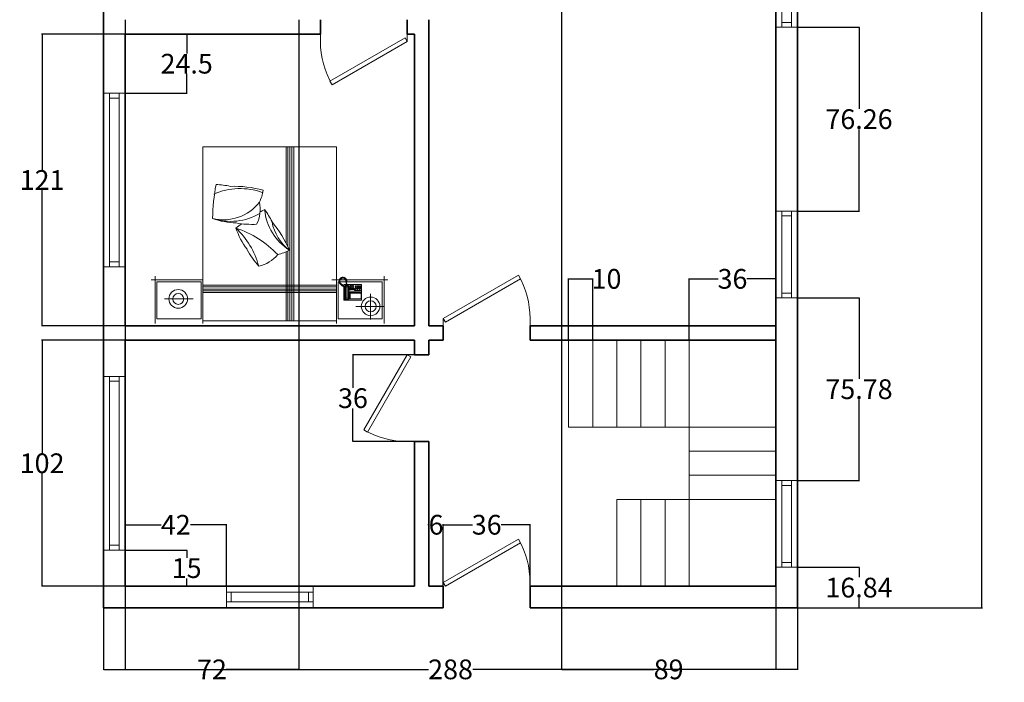
# Model space of a CAD drawing. Units: inches. Extents: x -254 to 1961, y 86 to 3025.
# Tile 2 of 6: x 117 to 525, y 133 to 408. Entities that reach past the tile are written whole.
import ezdxf

# ---------------------------------------------------------------- set-up
doc = ezdxf.new("R2010")
doc.units = ezdxf.units.IN
doc.header["$MEASUREMENT"] = 0
for name, color, linetype, lineweight in [('A-ANNO-DIMS', 2, 'Continuous', 18), ('DOORS', 40, 'Continuous', 18), ('FURNITURE', 151, 'Continuous', 13), ('STAIRCASE', 212, 'Continuous', 18), ('WALLS', 255, 'Continuous', 35), ('WINDOWS', 50, 'Continuous', 18)]:
    doc.layers.add(name, color=color, linetype=linetype, lineweight=lineweight)
doc.styles.get("Standard").update_dxf_attribs({"font": 'arial.ttf'})
doc.dimstyles.get("Standard").update_dxf_attribs({"dimtxt": 8.18, "dimasz": 0.18, "dimexe": 0.18, "dimexo": 0.0625, "dimgap": 0.09, "dimtad": 0, "dimtih": 1, "dimtoh": 1, "dimdec": 1, "dimzin": 0, "dimdsep": 46, "dimlunit": 3, "dimtxsty": 'Standard', "dimcen": 0.09, "dimadec": 0, "dimazin": 0, "dimtfac": 1, "dimtdec": 1, "dimtofl": 0, "dimtmove": 0, "dimatfit": 3, "dimfxl": 1, "dimtolj": 1, "dimtzin": 0, "dimarcsym": 0})

# ---------------------------------------------------------------- blocks, each defined once
blk = doc.blocks.new('*U5')
for p, q in [((0, 0), (0, -6)), ((36, 0), (36, -6))]:
    blk.add_line(p, q)
blk.add_lwpolyline([(0, 0), (31.18, 18), (32.05, 16.48), (0.87, -1.52)], close=True)
blk.add_arc((0, 0), 36, 0, 30)
blk = doc.blocks.new('*U3')
for p, q in [((-36, 0), (-36, 6)), ((0, 0), (0, 6))]:
    blk.add_line(p, q)
blk.add_lwpolyline([(0, 0), (-31.18, -18), (-32.05, -16.48), (-0.88, 1.52)], close=True)
blk.add_arc((0, 0), 36, 180, 210)
blk = doc.blocks.new('*U7')
for p, q in [((0, 0), (0, -6)), ((-36, 0), (-36, -6))]:
    blk.add_line(p, q)
blk.add_lwpolyline([(0, 0), (-31.18, 18), (-32.05, 16.48), (-0.88, -1.52)], close=True)
blk.add_arc((0, 0), 36, 150, 180)
blk = doc.blocks.new('BED-DOUBLE-NIGHTSTANDS')
for p, q in [((1.58, 73.32), (1.58, 53.78)), ((20.68, 71.37), (2.35, 71.37)), ((2.35, 71.37), (2.35, 56.1)), ((20.68, 56.1), (20.68, 71.37)), ((21.4, 73.32), (21.4, 53.78)), ((76.84, 72.19), (21.4, 72.19)), ((21.4, 72.19), (21.4, 0)), ((55.98, 43.63), (55.98, 72.19)), ((56.73, 43.3), (56.73, 72.19)), ((57.47, 0), (57.47, 72.19)), ((58.37, 0), (58.37, 72.19)), ((59.13, 0), (59.13, 72.19)), ((76.84, 73.32), (76.84, 53.78)), ((76.84, 0), (76.84, 72.19)), ((77.56, 56.1), (77.56, 71.37)), ((77.56, 71.37), (95.89, 71.37)), ((91.03, 61.02), (91.03, 71.64)), ((95.89, 71.37), (95.89, 56.1)), ((96.61, 73.32), (96.61, 53.78)), ((96.71, 66.24), (84.84, 66.24)), ((5.54, 63.15), (17.4, 63.15)), ((79.99, 63.51), (80.08, 63.61)), ((79.99, 57.27), (79.99, 63.51)), ((80.08, 63.61), (87.23, 63.61)), ((80.58, 63.47), (80.35, 63.24)), ((80.35, 63.24), (80.35, 57.81)), ((80.49, 63.33), (80.44, 63.15)), ((80.85, 62.75), (80.44, 63.15)), ((80.44, 63.15), (80.44, 61.93)), ((80.44, 61.93), (80.54, 61.7)), ((80.67, 63.42), (80.49, 63.33)), ((80.54, 61.7), (80.67, 61.48)), ((81.94, 63.47), (80.58, 63.47)), ((81.76, 63.42), (80.67, 63.42)), ((80.9, 62.84), (80.67, 63.42)), ((80.67, 61.48), (80.72, 61.16)), ((80.9, 62.84), (80.85, 62.75)), ((80.85, 62.75), (80.85, 60.71)), ((81.53, 62.84), (80.9, 62.84)), ((81.76, 63.42), (81.53, 62.84)), ((81.58, 62.75), (81.53, 62.84)), ((81.98, 63.15), (81.58, 62.75)), ((81.58, 62.75), (81.58, 60.71)), ((81.71, 61.16), (81.76, 61.48)), ((81.94, 63.33), (81.76, 63.42)), ((81.76, 61.48), (81.89, 61.7)), ((81.89, 61.7), (81.98, 61.93)), ((82.12, 63.24), (81.94, 63.47)), ((81.98, 63.15), (81.94, 63.33)), ((81.98, 61.93), (81.98, 63.15)), ((82.12, 57.77), (82.12, 63.24)), ((82.53, 60.71), (82.53, 63.11)), ((82.53, 63.11), (87.05, 63.11)), ((87.05, 63.11), (87.05, 60.71)), ((87.23, 63.61), (87.32, 63.51)), ((87.32, 63.51), (87.32, 57.27)), ((21.4, 60.55), (76.84, 60.55)), ((21.4, 59.81), (76.84, 59.81)), ((21.4, 59.06), (76.84, 59.06)), ((21.4, 58.17), (76.84, 58.17)), ((21.4, 57.41), (76.84, 57.41)), ((79.19, 57.22), (78.6, 56.71)), ((78.72, 57.24), (78.93, 57.44)), ((78.77, 56.95), (78.72, 57.24)), ((78.93, 57.44), (79.18, 57.31)), ((79.08, 57.58), (79.2, 57.7)), ((79.18, 57.31), (79.08, 57.58)), ((79.56, 57.55), (79.19, 57.22)), ((79.2, 57.7), (79.31, 57.62)), ((79.25, 57.75), (79.33, 57.83)), ((79.31, 57.62), (79.25, 57.75)), ((79.33, 57.83), (79.5, 57.77)), ((79.56, 57.64), (79.47, 57.65)), ((79.47, 57.65), (79.56, 57.55)), ((79.5, 57.77), (79.59, 57.85)), ((79.61, 57.7), (79.56, 57.64)), ((79.59, 57.85), (79.72, 57.98)), ((79.79, 57.85), (79.61, 57.7)), ((79.72, 57.98), (79.99, 58.08)), ((79.99, 57.9), (79.79, 57.85)), ((80.08, 57.18), (79.99, 57.27)), ((80.35, 57.81), (80.58, 57.54)), ((80.54, 59.31), (80.44, 59.08)), ((80.44, 59.08), (80.44, 57.86)), ((80.44, 57.86), (80.85, 58.26)), ((80.49, 57.68), (80.44, 57.86)), ((80.67, 57.59), (80.49, 57.68)), ((80.67, 59.53), (80.54, 59.31)), ((80.58, 57.54), (81.11, 57.54)), ((80.72, 59.85), (80.67, 59.53)), ((80.67, 57.59), (80.9, 58.17)), ((81.11, 57.59), (80.67, 57.59)), ((80.72, 61.16), (80.72, 60.71)), ((80.72, 60.71), (80.72, 59.85)), ((80.85, 60.71), (80.85, 58.26)), ((80.85, 58.26), (80.9, 58.17)), ((80.9, 58.17), (81.53, 58.17)), ((81.03, 57.07), (81.1, 57.36)), ((81.1, 57.36), (81.12, 57.72)), ((81.12, 57.72), (81.26, 57.72)), ((81.25, 57.33), (81.14, 56.87)), ((81.26, 57.72), (81.25, 57.33)), ((81.76, 57.59), (81.26, 57.59)), ((81.26, 57.54), (81.89, 57.54)), ((81.58, 58.26), (81.53, 58.17)), ((81.53, 58.17), (81.76, 57.59)), ((81.58, 60.71), (81.58, 58.26)), ((81.98, 57.86), (81.58, 58.26)), ((81.71, 60.71), (81.71, 61.16)), ((81.71, 59.85), (81.71, 60.71)), ((82.12, 60.34), (81.71, 60.34)), ((81.76, 59.53), (81.71, 59.85)), ((81.89, 59.31), (81.76, 59.53)), ((81.76, 57.59), (81.94, 57.68)), ((81.98, 59.08), (81.89, 59.31)), ((81.89, 57.54), (82.12, 57.77)), ((81.94, 57.68), (81.98, 57.86)), ((81.98, 57.86), (81.98, 59.08)), ((87.05, 60.71), (82.53, 60.71)), ((82.53, 60.17), (82.53, 60.62)), ((82.53, 60.62), (86.87, 60.62)), ((86.87, 60.34), (82.53, 60.34)), ((86.87, 60.17), (82.53, 60.17)), ((82.89, 59.44), (82.53, 59.44)), ((82.53, 59.44), (82.53, 59.17)), ((82.53, 59.17), (82.89, 59.17)), ((82.89, 58.94), (82.53, 58.94)), ((82.53, 58.94), (82.53, 58.67)), ((82.53, 58.67), (82.89, 58.67)), ((82.53, 58.45), (82.53, 58.17)), ((82.89, 58.45), (82.53, 58.45)), ((82.53, 58.17), (82.89, 58.17)), ((82.53, 57.9), (82.53, 57.63)), ((82.89, 57.9), (82.53, 57.9)), ((82.53, 57.63), (82.89, 57.63)), ((82.89, 59.17), (82.89, 59.44)), ((82.89, 58.67), (82.89, 58.94)), ((82.89, 58.17), (82.89, 58.45)), ((82.89, 57.63), (82.89, 57.9)), ((83.07, 59.44), (83.07, 59.17)), ((83.43, 59.44), (83.07, 59.44)), ((83.07, 59.17), (83.43, 59.17)), ((83.43, 58.94), (83.07, 58.94)), ((83.07, 58.94), (83.07, 58.67)), ((83.07, 58.67), (83.43, 58.67)), ((83.07, 58.4), (83.07, 58.13)), ((83.43, 58.4), (83.07, 58.4)), ((83.07, 58.13), (83.43, 58.13)), ((83.43, 57.9), (83.07, 57.9)), ((83.07, 57.9), (83.07, 57.63)), ((83.07, 57.63), (83.43, 57.63)), ((83.43, 59.17), (83.43, 59.44)), ((83.43, 58.67), (83.43, 58.94)), ((83.43, 58.13), (83.43, 58.4)), ((83.43, 57.63), (83.43, 57.9)), ((83.97, 59.44), (83.61, 59.44)), ((83.61, 59.44), (83.61, 59.17)), ((83.61, 59.17), (83.97, 59.17)), ((83.97, 58.94), (83.61, 58.94)), ((83.61, 58.94), (83.61, 58.67)), ((83.61, 58.67), (83.97, 58.67)), ((83.97, 58.4), (83.61, 58.4)), ((83.61, 58.4), (83.61, 58.13)), ((83.61, 58.13), (83.97, 58.13)), ((83.97, 57.9), (83.61, 57.9)), ((83.61, 57.9), (83.61, 57.63)), ((83.61, 57.63), (83.97, 57.63)), ((83.97, 59.17), (83.97, 59.44)), ((83.97, 58.67), (83.97, 58.94)), ((83.97, 58.13), (83.97, 58.4)), ((83.97, 57.63), (83.97, 57.9)), ((84.38, 58.85), (84.38, 59.67)), ((84.38, 59.67), (87.05, 59.67)), ((87.05, 58.85), (84.38, 58.85)), ((84.73, 60.17), (84.56, 60.34)), ((84.65, 58.45), (84.65, 58.63)), ((84.65, 58.63), (85.11, 58.63)), ((85.11, 58.45), (84.65, 58.45)), ((85.11, 57.95), (84.65, 57.95)), ((84.65, 57.95), (84.65, 57.68)), ((84.65, 57.68), (85.11, 57.68)), ((84.7, 60.62), (84.7, 60.17)), ((84.83, 59.44), (84.83, 59.58)), ((84.83, 59.58), (84.97, 59.58)), ((84.97, 59.44), (84.83, 59.44)), ((84.83, 58.94), (84.83, 59.08)), ((84.83, 59.08), (84.97, 59.08)), ((84.97, 58.94), (84.83, 58.94)), ((84.97, 59.58), (84.97, 59.44)), ((84.97, 59.08), (84.97, 58.94)), ((85.06, 60.62), (85.06, 60.17)), ((85.11, 58.63), (85.11, 58.45)), ((85.11, 57.68), (85.11, 57.95)), ((86.04, 58.85), (85.23, 59.67)), ((85.29, 58.63), (85.74, 58.63)), ((85.29, 58.45), (85.29, 58.63)), ((85.74, 58.45), (85.29, 58.45)), ((85.29, 57.95), (85.29, 57.68)), ((85.74, 57.95), (85.29, 57.95)), ((85.29, 57.68), (85.74, 57.68)), ((85.42, 60.62), (85.42, 60.17)), ((85.65, 59.44), (85.65, 59.58)), ((85.65, 59.58), (85.79, 59.58)), ((85.79, 59.44), (85.65, 59.44)), ((85.65, 58.94), (85.65, 59.08)), ((85.65, 59.08), (85.79, 59.08)), ((85.79, 58.94), (85.65, 58.94)), ((85.74, 58.63), (85.74, 58.45)), ((85.74, 57.68), (85.74, 57.95)), ((85.79, 60.62), (85.79, 60.17)), ((85.79, 59.58), (85.79, 59.44)), ((85.79, 59.08), (85.79, 58.94)), ((85.92, 58.63), (86.37, 58.63)), ((85.92, 58.45), (85.92, 58.63)), ((86.37, 58.45), (85.92, 58.45)), ((85.92, 57.95), (85.92, 57.68)), ((86.37, 57.95), (85.92, 57.95)), ((85.92, 57.68), (86.37, 57.68)), ((86.15, 60.62), (86.15, 60.17)), ((86.37, 58.52), (86.27, 58.63)), ((86.37, 58.63), (86.37, 58.45)), ((86.37, 57.68), (86.37, 57.95)), ((86.46, 59.44), (86.46, 59.58)), ((86.46, 59.58), (86.6, 59.58)), ((86.6, 59.44), (86.46, 59.44)), ((86.46, 58.94), (86.46, 59.08)), ((86.46, 59.08), (86.6, 59.08)), ((86.6, 58.94), (86.46, 58.94)), ((86.51, 60.62), (86.51, 60.17)), ((86.55, 58.63), (87.01, 58.63)), ((86.55, 58.45), (86.55, 58.63)), ((87.01, 58.45), (86.55, 58.45)), ((86.55, 57.95), (86.55, 57.68)), ((87.01, 57.95), (86.55, 57.95)), ((86.55, 57.68), (87.01, 57.68)), ((86.6, 59.58), (86.6, 59.44)), ((86.6, 59.08), (86.6, 58.94)), ((86.87, 60.62), (86.87, 60.17)), ((87.01, 57.89), (86.95, 57.95)), ((87.01, 58.63), (87.01, 58.45)), ((87.01, 57.68), (87.01, 57.95)), ((87.05, 59.67), (87.05, 58.85)), ((87.32, 57.27), (87.23, 57.18)), ((0, 55.17), (21.4, 55.17)), ((2.35, 56.1), (20.68, 56.1)), ((98.24, 55.17), (74.88, 55.17)), ((95.89, 56.1), (77.56, 56.1)), ((77.91, 55.74), (77.96, 55.97)), ((78.19, 55.65), (77.91, 55.74)), ((77.96, 55.97), (78.2, 55.97)), ((77.96, 55.52), (78.19, 55.65)), ((77.99, 55.33), (77.96, 55.52)), ((78.28, 55.34), (77.99, 55.33)), ((78.01, 56.15), (78.07, 56.36)), ((78.2, 55.97), (78.01, 56.15)), ((78.06, 55.09), (78.28, 55.34)), ((78.13, 54.91), (78.06, 55.09)), ((78.07, 56.36), (78.37, 56.35)), ((78.1, 56.45), (78.18, 56.73)), ((78.37, 56.35), (78.1, 56.45)), ((78.4, 54.99), (78.13, 54.91)), ((78.18, 56.73), (78.46, 56.7)), ((78.38, 55.31), (78.24, 55.31)), ((78.27, 54.75), (78.4, 54.99)), ((78.39, 54.64), (78.27, 54.75)), ((78.59, 56.7), (78.29, 55.84)), ((78.29, 55.84), (78.41, 55.15)), ((78.39, 56.9), (78.56, 57.08)), ((78.46, 56.7), (78.39, 56.9)), ((78.64, 54.75), (78.39, 54.64)), ((78.41, 55.15), (78.82, 54.76)), ((78.53, 54.5), (78.64, 54.75)), ((78.68, 54.37), (78.53, 54.5)), ((78.56, 57.08), (78.77, 56.95)), ((78.87, 54.61), (78.68, 54.37)), ((78.82, 54.76), (79.35, 54.53)), ((78.84, 54.33), (78.87, 54.61)), ((78.99, 54.26), (78.84, 54.33)), ((79.2, 54.44), (78.99, 54.26)), ((79.21, 54.2), (79.2, 54.44)), ((79.38, 54.15), (79.21, 54.2)), ((79.35, 54.53), (79.9, 54.57)), ((79.49, 54.44), (79.38, 54.15)), ((79.55, 54.18), (79.49, 54.44)), ((79.71, 54.2), (79.55, 54.18)), ((79.82, 54.44), (79.71, 54.2)), ((79.93, 54.2), (79.82, 54.44)), ((79.9, 54.57), (80.38, 54.83)), ((80.13, 54.25), (79.93, 54.2)), ((81.06, 57.18), (80.08, 57.18)), ((80.32, 54.37), (80.1, 54.55)), ((80.1, 54.55), (80.13, 54.25)), ((80.49, 54.48), (80.32, 54.37)), ((80.38, 54.83), (80.73, 55.27)), ((80.67, 54.57), (80.46, 54.73)), ((80.46, 54.73), (80.49, 54.48)), ((80.8, 54.74), (80.67, 54.57)), ((80.95, 54.94), (80.68, 54.99)), ((80.68, 54.99), (80.8, 54.74)), ((80.73, 55.27), (80.78, 55.85)), ((80.74, 56.06), (80.9, 56.18)), ((80.78, 55.85), (80.74, 56.06)), ((81.11, 55.38), (80.81, 55.35)), ((80.81, 55.35), (81.07, 55.15)), ((81.13, 55.83), (80.87, 55.78)), ((80.87, 55.78), (81.12, 55.63)), ((80.9, 56.41), (80.92, 56.63)), ((80.9, 56.18), (80.9, 56.41)), ((80.92, 56.63), (81.03, 57.07)), ((81.07, 55.15), (80.95, 54.94)), ((81.04, 56.2), (81.01, 56.15)), ((81.01, 56.15), (81.12, 56.05)), ((81.14, 56.87), (81.03, 56.44)), ((81.03, 56.44), (81.04, 56.2)), ((81.12, 55.63), (81.11, 55.38)), ((81.12, 56.05), (81.13, 55.83)), ((87.23, 57.18), (81.22, 57.18)), ((56.73, 0), (56.73, 41.48)), ((55.98, 0), (55.98, 39.96)), ((21.4, 0), (76.84, 0))]:
    blk.add_line(p, q)
for centre, radius in [((91.03, 66.24), 3.87), ((11.21, 63.15), 3.87), ((11.21, 63.15), 2.29), ((91.03, 66.24), 2.29)]:
    blk.add_circle(centre, radius)
for centre, radius, start, end in [((11.42, 58.69), 34.44, 313.5807, 344.664), ((74.12, 23.89), 39.12, 138.9434, 151.5029), ((41.57, 35.76), 14.16, 39.5375, 77.5218), ((21.54, 74.27), 42.76, 288.5712, 316.3694), ((64.75, 23.92), 31.18, 143.3149, 161.6473), ((69.36, 24.04), 22.39, 122.3105, 174.6609), ((14.94, 61.05), 46.14, 319.6791, 336.9358), ((69.1, 27.6), 19.32, 127.3136, 169.3014), ((47.53, 23.64), 21.7, 62.9638, 76.7966), ((87.82, 103.02), 87.02, 232.7582, 234.7034), ((36.16, 0.49), 31.18, 91.7513, 110.0837), ((32.98, 6.89), 24.09, 59.8649, 108.19), ((29.97, 11.42), 18.9, 37.9983, 103.8151), ((112.46, 31.59), 87.02, 181.1946, 190.5116), ((41.96, -6.88), 39.12, 87.3798, 99.9393), ((31.02, 26.01), 14.16, 347.9738, 25.9582), ((23.83, 43.59), 29.07, 323.0649, 334.741), ((87.82, 103.02), 87.02, 240.6207, 242.0752), ((25.24, 13.81), 21.7, 11.4002, 25.233), ((36.91, 44.65), 27.26, 246.3586, 289.7064), ((26.13, 44.77), 29.07, 271.5012, 283.1774), ((34.28, 62.58), 46.14, 268.1155, 285.3722)]:
    blk.add_arc(centre, radius, start, end)
blk = doc.blocks.new('WIN-36IN')
for p, q in [((2.5, 35), (2.5, 2)), ((6.5, 35), (6.5, 2))]:
    blk.add_line(p, q)
for points in [[(0, 36), (9, 36), (9, 0), (0, 0)], [(2.5, 36), (6.5, 36), (6.5, 34), (2.5, 34)], [(2.5, 0), (6.5, 0), (6.5, 2), (2.5, 2)]]:
    blk.add_lwpolyline(points, close=True)
blk = doc.blocks.new('WIN-72IN')
for p, q in [((2.5, 70), (2.5, 2)), ((6.5, 70), (6.5, 2))]:
    blk.add_line(p, q)
for points in [[(0, 72), (9, 72), (9, 0), (0, 0)], [(2.5, 72), (6.5, 72), (6.5, 70), (2.5, 70)], [(2.5, 0), (6.5, 0), (6.5, 2), (2.5, 2)]]:
    blk.add_lwpolyline(points, close=True)
blk = doc.blocks.new('*D22')
at = {"layer": 'A-ANNO-DIMS', "color": 0, "lineweight": -2, "transparency": 16777216}
for p, q in [((151.38, 163.93), (151.38, 138.31)), ((439.38, 163.93), (439.38, 138.31)), ((151.56, 138.49), (286.18, 138.49)), ((439.2, 138.49), (304.59, 138.49))]:
    blk.add_line(p, q, dxfattribs=at)
at = {"layer": 'A-ANNO-DIMS', "color": 0, "transparency": 16777216}
for points in [[(151.56, 138.52), (151.56, 138.46), (151.38, 138.49)], [(439.2, 138.52), (439.2, 138.46), (439.38, 138.49)]]:
    blk.add_solid(points, dxfattribs=at)
at = {"layer": 'Defpoints', "color": 0, "transparency": 16777216}
for p in [(151.38, 163.99), (439.38, 163.99), (439.38, 138.49)]:
    blk.add_point(p, dxfattribs=at)
at = {"layer": 'A-ANNO-DIMS', "color": 0, "transparency": 16777216, "insert": (295.38, 138.49), "char_height": 8.18, "attachment_point": 5}
blk.add_mtext('\\A1;288', dxfattribs=at)
blk = doc.blocks.new('*D23')
at = {"layer": 'A-ANNO-DIMS', "color": 0, "lineweight": -2, "transparency": 16777216}
for p, q in [((439.44, 667.99), (516.06, 667.99)), ((515.88, 667.81), (515.88, 420.26)), ((515.88, 164.17), (515.88, 411.73)), ((439.44, 163.99), (516.06, 163.99))]:
    blk.add_line(p, q, dxfattribs=at)
at = {"layer": 'A-ANNO-DIMS', "color": 0, "transparency": 16777216}
for points in [[(515.85, 667.81), (515.91, 667.81), (515.88, 667.99)], [(515.85, 164.17), (515.91, 164.17), (515.88, 163.99)]]:
    blk.add_solid(points, dxfattribs=at)
at = {"layer": 'Defpoints', "color": 0, "transparency": 16777216}
for p in [(439.38, 667.99), (515.88, 667.99), (439.38, 163.99)]:
    blk.add_point(p, dxfattribs=at)
at = {"layer": 'A-ANNO-DIMS', "color": 0, "transparency": 16777216, "insert": (515.88, 415.99), "char_height": 8.18, "attachment_point": 5}
blk.add_mtext('\\A1;504', dxfattribs=at)
blk = doc.blocks.new('*D30')
at = {"layer": 'A-ANNO-DIMS', "color": 0, "lineweight": -2, "transparency": 16777216}
for p, q in [((160.32, 401.99), (125.7, 401.99)), ((125.88, 401.81), (125.88, 345.69)), ((125.88, 281.17), (125.88, 337.3)), ((160.32, 280.99), (125.7, 280.99))]:
    blk.add_line(p, q, dxfattribs=at)
at = {"layer": 'A-ANNO-DIMS', "color": 0, "transparency": 16777216}
for points in [[(125.85, 401.81), (125.91, 401.81), (125.88, 401.99)], [(125.85, 281.17), (125.91, 281.17), (125.88, 280.99)]]:
    blk.add_solid(points, dxfattribs=at)
at = {"layer": 'Defpoints', "color": 0, "transparency": 16777216}
for p in [(125.88, 401.99), (160.38, 401.99), (160.38, 280.99)]:
    blk.add_point(p, dxfattribs=at)
at = {"layer": 'A-ANNO-DIMS', "color": 0, "transparency": 16777216, "insert": (125.88, 341.49), "char_height": 8.18, "attachment_point": 5}
blk.add_mtext('\\A1;121', dxfattribs=at)
blk = doc.blocks.new('*D31')
at = {"layer": 'A-ANNO-DIMS', "color": 0, "lineweight": -2, "transparency": 16777216}
for p, q in [((160.32, 274.99), (125.7, 274.99)), ((125.88, 274.81), (125.88, 228.26)), ((125.88, 173.17), (125.88, 219.73)), ((160.32, 172.99), (125.7, 172.99))]:
    blk.add_line(p, q, dxfattribs=at)
at = {"layer": 'A-ANNO-DIMS', "color": 0, "transparency": 16777216}
for points in [[(125.85, 274.81), (125.91, 274.81), (125.88, 274.99)], [(125.85, 173.17), (125.91, 173.17), (125.88, 172.99)]]:
    blk.add_solid(points, dxfattribs=at)
at = {"layer": 'Defpoints', "color": 0, "transparency": 16777216}
for p in [(125.88, 274.99), (160.38, 274.99), (160.38, 172.99)]:
    blk.add_point(p, dxfattribs=at)
at = {"layer": 'A-ANNO-DIMS', "color": 0, "transparency": 16777216, "insert": (125.88, 223.99), "char_height": 8.18, "attachment_point": 5}
blk.add_mtext('\\A1;102', dxfattribs=at)
blk = doc.blocks.new('*D32')
at = {"layer": 'A-ANNO-DIMS', "color": 0, "lineweight": -2, "transparency": 16777216}
for p, q in [((160.38, 173.06), (160.38, 198.67)), ((160.56, 198.49), (175.31, 198.49)), ((202.2, 198.49), (187.45, 198.49)), ((202.38, 173.06), (202.38, 198.67))]:
    blk.add_line(p, q, dxfattribs=at)
at = {"layer": 'A-ANNO-DIMS', "color": 0, "transparency": 16777216}
for points in [[(160.56, 198.52), (160.56, 198.46), (160.38, 198.49)], [(202.2, 198.52), (202.2, 198.46), (202.38, 198.49)]]:
    blk.add_solid(points, dxfattribs=at)
at = {"layer": 'Defpoints', "color": 0, "transparency": 16777216}
for p in [(202.38, 198.49), (160.38, 172.99), (202.38, 172.99)]:
    blk.add_point(p, dxfattribs=at)
at = {"layer": 'A-ANNO-DIMS', "color": 0, "transparency": 16777216, "insert": (181.38, 198.49), "char_height": 8.18, "attachment_point": 5}
blk.add_mtext('\\A1;42', dxfattribs=at)
blk = doc.blocks.new('*D33')
at = {"layer": 'A-ANNO-DIMS', "color": 0, "lineweight": -2, "transparency": 16777216}
for p, q in [((292.38, 173.06), (292.38, 198.67)), ((292.56, 198.49), (304.44, 198.49)), ((328.2, 198.49), (316.33, 198.49)), ((328.38, 173.06), (328.38, 198.67))]:
    blk.add_line(p, q, dxfattribs=at)
at = {"layer": 'A-ANNO-DIMS', "color": 0, "transparency": 16777216}
for points in [[(292.56, 198.52), (292.56, 198.46), (292.38, 198.49)], [(328.2, 198.52), (328.2, 198.46), (328.38, 198.49)]]:
    blk.add_solid(points, dxfattribs=at)
at = {"layer": 'Defpoints', "color": 0, "transparency": 16777216}
for p in [(328.38, 198.49), (292.38, 172.99), (328.38, 172.99)]:
    blk.add_point(p, dxfattribs=at)
at = {"layer": 'A-ANNO-DIMS', "color": 0, "transparency": 16777216, "insert": (310.38, 198.49), "char_height": 8.18, "attachment_point": 5}
blk.add_mtext('\\A1;36', dxfattribs=at)
blk = doc.blocks.new('*D34')
at = {"layer": 'A-ANNO-DIMS', "color": 0, "lineweight": -2, "transparency": 16777216}
for p, q in [((286.201832, 198.494989), (286.021832, 198.494989)), ((286.381832, 173.057489), (286.381832, 198.674989)), ((292.381832, 173.057489), (292.381832, 198.674989)), ((292.561832, 198.494989), (292.741832, 198.494989))]:
    blk.add_line(p, q, dxfattribs=at)
at = {"layer": 'A-ANNO-DIMS', "color": 0, "transparency": 16777216}
for points in [[(286.201832, 198.524989), (286.201832, 198.464989), (286.381832, 198.494989)], [(292.561832, 198.524989), (292.561832, 198.464989), (292.381832, 198.494989)]]:
    blk.add_solid(points, dxfattribs=at)
at = {"layer": 'Defpoints', "color": 0, "transparency": 16777216}
for p in [(292.381832, 198.494989), (286.381832, 172.994989), (292.381832, 172.994989)]:
    blk.add_point(p, dxfattribs=at)
at = {"layer": 'A-ANNO-DIMS', "color": 0, "transparency": 16777216, "insert": (289.381832, 198.494989), "char_height": 8.18, "attachment_point": 5}
blk.add_mtext('\\A1;6', dxfattribs=at)
blk = doc.blocks.new('*D35')
at = {"layer": 'A-ANNO-DIMS', "color": 0, "lineweight": -2, "transparency": 16777216}
for p, q in [((394.38, 275.06), (394.38, 300.67)), ((394.56, 300.49), (406.44, 300.49)), ((430.2, 300.49), (418.33, 300.49)), ((430.38, 275.06), (430.38, 300.67))]:
    blk.add_line(p, q, dxfattribs=at)
at = {"layer": 'A-ANNO-DIMS', "color": 0, "transparency": 16777216}
for points in [[(394.56, 300.52), (394.56, 300.46), (394.38, 300.49)], [(430.2, 300.52), (430.2, 300.46), (430.38, 300.49)]]:
    blk.add_solid(points, dxfattribs=at)
at = {"layer": 'Defpoints', "color": 0, "transparency": 16777216}
for p in [(430.38, 300.49), (394.38, 274.99), (430.38, 274.99)]:
    blk.add_point(p, dxfattribs=at)
at = {"layer": 'A-ANNO-DIMS', "color": 0, "transparency": 16777216, "insert": (412.38, 300.49), "char_height": 8.18, "attachment_point": 5}
blk.add_mtext('\\A1;36', dxfattribs=at)
blk = doc.blocks.new('*D36')
at = {"layer": 'A-ANNO-DIMS', "color": 0, "lineweight": -2, "transparency": 16777216}
for p, q in [((160.44, 187.99), (186.06, 187.99)), ((185.88, 187.81), (185.88, 184.76)), ((185.88, 173.17), (185.88, 176.23)), ((160.44, 172.99), (186.06, 172.99))]:
    blk.add_line(p, q, dxfattribs=at)
at = {"layer": 'A-ANNO-DIMS', "color": 0, "transparency": 16777216}
for points in [[(185.85, 187.81), (185.91, 187.81), (185.88, 187.99)], [(185.85, 173.17), (185.91, 173.17), (185.88, 172.99)]]:
    blk.add_solid(points, dxfattribs=at)
at = {"layer": 'Defpoints', "color": 0, "transparency": 16777216}
for p in [(160.38, 187.99), (160.38, 172.99), (185.88, 172.99)]:
    blk.add_point(p, dxfattribs=at)
at = {"layer": 'A-ANNO-DIMS', "color": 0, "transparency": 16777216, "insert": (185.88, 180.49), "char_height": 8.18, "attachment_point": 5}
blk.add_mtext('\\A1;15', dxfattribs=at)
blk = doc.blocks.new('*D37')
at = {"layer": 'A-ANNO-DIMS', "color": 0, "lineweight": -2, "transparency": 16777216}
for p, q in [((160.44, 401.99), (186.06, 401.99)), ((185.88, 401.81), (185.88, 394.01)), ((185.88, 377.67), (185.88, 385.48)), ((160.44, 377.49), (186.06, 377.49))]:
    blk.add_line(p, q, dxfattribs=at)
at = {"layer": 'A-ANNO-DIMS', "color": 0, "transparency": 16777216}
for points in [[(185.85, 401.81), (185.91, 401.81), (185.88, 401.99)], [(185.85, 377.67), (185.91, 377.67), (185.88, 377.49)]]:
    blk.add_solid(points, dxfattribs=at)
at = {"layer": 'Defpoints', "color": 0, "transparency": 16777216}
for p in [(160.38, 401.99), (160.38, 377.49), (185.88, 377.49)]:
    blk.add_point(p, dxfattribs=at)
at = {"layer": 'A-ANNO-DIMS', "color": 0, "transparency": 16777216, "insert": (185.88, 389.74), "char_height": 8.18, "attachment_point": 5}
blk.add_mtext('\\A1;24.5', dxfattribs=at)
blk = doc.blocks.new('*D41')
at = {"layer": 'A-ANNO-DIMS', "color": 0, "lineweight": -2, "transparency": 16777216}
for p, q in [((439.44, 404.87), (465.06, 404.87)), ((464.88, 404.69), (464.88, 371)), ((464.88, 328.79), (464.88, 362.47)), ((439.44, 328.61), (465.06, 328.61))]:
    blk.add_line(p, q, dxfattribs=at)
at = {"layer": 'A-ANNO-DIMS', "color": 0, "transparency": 16777216}
for points in [[(464.85, 404.69), (464.91, 404.69), (464.88, 404.87)], [(464.85, 328.79), (464.91, 328.79), (464.88, 328.61)]]:
    blk.add_solid(points, dxfattribs=at)
at = {"layer": 'Defpoints', "color": 0, "transparency": 16777216}
for p in [(439.38, 404.87), (439.38, 328.61), (464.88, 328.61)]:
    blk.add_point(p, dxfattribs=at)
at = {"layer": 'A-ANNO-DIMS', "color": 0, "transparency": 16777216, "insert": (464.88, 366.74), "char_height": 8.18, "attachment_point": 5}
blk.add_mtext('\\A1;76.26', dxfattribs=at)
blk = doc.blocks.new('*D42')
at = {"layer": 'A-ANNO-DIMS', "color": 0, "lineweight": -2, "transparency": 16777216}
for p, q in [((439.44, 292.61), (465.06, 292.61)), ((464.88, 292.43), (464.88, 258.99)), ((464.88, 217.01), (464.88, 250.46)), ((439.44, 216.83), (465.06, 216.83))]:
    blk.add_line(p, q, dxfattribs=at)
at = {"layer": 'A-ANNO-DIMS', "color": 0, "transparency": 16777216}
for points in [[(464.85, 292.43), (464.91, 292.43), (464.88, 292.61)], [(464.85, 217.01), (464.91, 217.01), (464.88, 216.83)]]:
    blk.add_solid(points, dxfattribs=at)
at = {"layer": 'Defpoints', "color": 0, "transparency": 16777216}
for p in [(439.38, 292.61), (439.38, 216.83), (464.88, 216.83)]:
    blk.add_point(p, dxfattribs=at)
at = {"layer": 'A-ANNO-DIMS', "color": 0, "transparency": 16777216, "insert": (464.88, 254.72), "char_height": 8.18, "attachment_point": 5}
blk.add_mtext('\\A1;75.78', dxfattribs=at)
blk = doc.blocks.new('*D43')
at = {"layer": 'A-ANNO-DIMS', "color": 0, "lineweight": -2, "transparency": 16777216}
for p, q in [((439.44, 180.83), (465.06, 180.83)), ((464.88, 180.65), (464.88, 176.68)), ((464.88, 164.17), (464.88, 168.15)), ((439.44, 163.99), (465.06, 163.99))]:
    blk.add_line(p, q, dxfattribs=at)
at = {"layer": 'A-ANNO-DIMS', "color": 0, "transparency": 16777216}
for points in [[(464.85, 180.65), (464.91, 180.65), (464.88, 180.83)], [(464.85, 164.17), (464.91, 164.17), (464.88, 163.99)]]:
    blk.add_solid(points, dxfattribs=at)
at = {"layer": 'Defpoints', "color": 0, "transparency": 16777216}
for p in [(439.38, 180.83), (439.38, 163.99), (464.88, 163.99)]:
    blk.add_point(p, dxfattribs=at)
at = {"layer": 'A-ANNO-DIMS', "color": 0, "transparency": 16777216, "insert": (464.88, 172.41), "char_height": 8.18, "attachment_point": 5}
blk.add_mtext('\\A1;16.84', dxfattribs=at)
blk = doc.blocks.new('*D44')
at = {"layer": 'A-ANNO-DIMS', "color": 0, "lineweight": -2, "transparency": 16777216}
for p, q in [((344.38, 275.06), (344.38, 300.67)), ((344.56, 300.49), (354.2, 300.49)), ((354.38, 275.06), (354.38, 300.67)), ((354.38, 300.49), (354.56, 300.49))]:
    blk.add_line(p, q, dxfattribs=at)
at = {"layer": 'A-ANNO-DIMS', "color": 0, "transparency": 16777216}
for points in [[(344.56, 300.52), (344.56, 300.46), (344.38, 300.49)], [(354.2, 300.52), (354.2, 300.46), (354.38, 300.49)]]:
    blk.add_solid(points, dxfattribs=at)
at = {"layer": 'Defpoints', "color": 0, "transparency": 16777216}
for p in [(354.38, 300.49), (344.38, 274.99), (354.38, 274.99)]:
    blk.add_point(p, dxfattribs=at)
at = {"layer": 'A-ANNO-DIMS', "color": 0, "transparency": 16777216, "insert": (360.11, 300.49), "char_height": 8.18, "attachment_point": 5}
blk.add_mtext('\\A1;10', dxfattribs=at)
blk = doc.blocks.new('*D45')
at = {"layer": 'A-ANNO-DIMS', "color": 0, "lineweight": -2, "transparency": 16777216}
for p, q in [((280.32, 268.99), (254.7, 268.99)), ((254.88, 268.81), (254.88, 255.26)), ((254.88, 233.17), (254.88, 246.73)), ((280.32, 232.99), (254.7, 232.99))]:
    blk.add_line(p, q, dxfattribs=at)
at = {"layer": 'A-ANNO-DIMS', "color": 0, "transparency": 16777216}
for points in [[(254.85, 268.81), (254.91, 268.81), (254.88, 268.99)], [(254.85, 233.17), (254.91, 233.17), (254.88, 232.99)]]:
    blk.add_solid(points, dxfattribs=at)
at = {"layer": 'Defpoints', "color": 0, "transparency": 16777216}
for p in [(254.88, 268.99), (280.38, 268.99), (280.38, 232.99)]:
    blk.add_point(p, dxfattribs=at)
at = {"layer": 'A-ANNO-DIMS', "color": 0, "transparency": 16777216, "insert": (254.88, 250.99), "char_height": 8.18, "attachment_point": 5}
blk.add_mtext('\\A1;36', dxfattribs=at)
blk = doc.blocks.new('*D46')
at = {"layer": 'A-ANNO-DIMS', "color": 0, "lineweight": -2, "transparency": 16777216}
for p, q in [((160.38, 407.93), (160.38, 138.31)), ((232.38, 407.93), (232.38, 138.31)), ((160.56, 138.49), (190.51, 138.49)), ((232.2, 138.49), (202.26, 138.49))]:
    blk.add_line(p, q, dxfattribs=at)
at = {"layer": 'A-ANNO-DIMS', "color": 0, "transparency": 16777216}
for points in [[(160.56, 138.52), (160.56, 138.46), (160.38, 138.49)], [(232.2, 138.52), (232.2, 138.46), (232.38, 138.49)]]:
    blk.add_solid(points, dxfattribs=at)
at = {"layer": 'Defpoints', "color": 0, "transparency": 16777216}
for p in [(160.38, 407.99), (232.38, 407.99), (232.38, 138.49)]:
    blk.add_point(p, dxfattribs=at)
at = {"layer": 'A-ANNO-DIMS', "color": 0, "transparency": 16777216, "insert": (196.38, 138.49), "char_height": 8.18, "attachment_point": 5}
blk.add_mtext('\\A1;72', dxfattribs=at)
blk = doc.blocks.new('*D48')
at = {"layer": 'A-ANNO-DIMS', "color": 0, "lineweight": -2, "transparency": 16777216}
for p, q in [((341.38, 457.93), (341.38, 138.31)), ((430.38, 457.93), (430.38, 138.31)), ((341.56, 138.49), (379.92, 138.49)), ((430.2, 138.49), (391.84, 138.49))]:
    blk.add_line(p, q, dxfattribs=at)
at = {"layer": 'A-ANNO-DIMS', "color": 0, "transparency": 16777216}
for points in [[(341.56, 138.52), (341.56, 138.46), (341.38, 138.49)], [(430.2, 138.52), (430.2, 138.46), (430.38, 138.49)]]:
    blk.add_solid(points, dxfattribs=at)
at = {"layer": 'Defpoints', "color": 0, "transparency": 16777216}
for p in [(341.38, 457.99), (430.38, 457.99), (430.38, 138.49)]:
    blk.add_point(p, dxfattribs=at)
at = {"layer": 'A-ANNO-DIMS', "color": 0, "transparency": 16777216, "insert": (385.88, 138.49), "char_height": 8.18, "attachment_point": 5}
blk.add_mtext('\\A1;89', dxfattribs=at)

msp = doc.modelspace()

# ---------------------------------------------------------------- linework, layer by layer
at = {"layer": 'STAIRCASE'}
for p, q in [((430.3818, 274.995), (344.3818, 274.995)), ((354.3818, 238.995), (354.3818, 274.995)), ((364.3818, 238.995), (364.3818, 274.995)), ((374.3818, 238.995), (374.3818, 274.995)), ((384.3818, 238.995), (384.3818, 274.995)), ((394.3818, 238.995), (394.3818, 274.995)), ((430.3818, 172.995), (430.3818, 274.995)), ((394.3818, 238.995), (430.3818, 238.995)), ((394.3818, 228.995), (430.3818, 228.995)), ((394.3818, 218.995), (430.3818, 218.995)), ((374.3818, 172.995), (374.3818, 208.995)), ((384.3818, 172.995), (384.3818, 208.995)), ((394.3818, 172.995), (394.3818, 208.995)), ((394.3818, 208.995), (430.3818, 208.995)), ((364.3818, 172.995), (430.3818, 172.995))]:
    msp.add_line(p, q, dxfattribs=at)
msp.add_lwpolyline([(364.3818, 172.995), (364.3818, 208.995), (394.3818, 208.995), (394.3818, 238.995), (344.3818, 238.995), (344.3818, 274.995)], dxfattribs=at)
at = {"layer": 'WALLS'}
for p, q in [((151.3818, 163.995), (151.3818, 667.995)), ((439.3818, 163.995), (439.3818, 667.995)), ((430.3818, 280.995), (430.3818, 451.995)), ((241.3818, 401.995), (241.3818, 407.995)), ((277.3818, 401.995), (277.3818, 407.995)), ((286.3818, 280.995), (286.3818, 407.995)), ((160.3818, 401.995), (241.3818, 401.995)), ((160.3818, 280.995), (160.3818, 401.995)), ((277.3818, 401.995), (280.3818, 401.995)), ((280.3818, 280.995), (280.3818, 401.995)), ((160.3818, 280.995), (280.3818, 280.995)), ((286.3818, 280.995), (292.3818, 280.995)), ((292.3818, 274.995), (292.3818, 280.995)), ((328.3818, 280.995), (430.3818, 280.995)), ((328.3818, 274.995), (328.3818, 280.995)), ((160.3818, 172.995), (160.3818, 274.995)), ((160.3818, 274.995), (280.3818, 274.995)), ((280.3818, 268.995), (280.3818, 274.995)), ((286.3818, 268.995), (286.3818, 274.995)), ((286.3818, 274.995), (292.3818, 274.995)), ((328.3818, 274.995), (430.3818, 274.995)), ((430.3818, 172.995), (430.3818, 274.995)), ((280.3818, 268.995), (286.3818, 268.995)), ((280.3818, 172.995), (280.3818, 232.995)), ((280.3818, 232.995), (286.3818, 232.995)), ((286.3818, 172.995), (286.3818, 232.995)), ((160.3818, 172.995), (280.3818, 172.995)), ((286.3818, 172.995), (292.3818, 172.995)), ((292.3818, 163.995), (292.3818, 172.995)), ((328.3818, 163.995), (328.3818, 172.995)), ((328.3818, 172.995), (430.3818, 172.995)), ((151.3818, 163.995), (292.3818, 163.995)), ((328.3818, 163.995), (439.3818, 163.995))]:
    msp.add_line(p, q, dxfattribs=at)

# ---------------------------------------------------------------- block references
at = {"layer": 'DOORS'}
for name, p in [('*U3', (277.3818, 398.995)), ('*U5', (292.3818, 283.995)), ('*U5', (292.3818, 174.495))]:
    msp.add_blockref(name, p, dxfattribs=at)
at = {"layer": 'DOORS', "rotation": 90}
msp.add_blockref('*U7', (277.3818, 268.995), dxfattribs=at)
at = {"layer": 'FURNITURE', "extrusion": (0, 0, -1), "zscale": -1, "rotation": 180}
msp.add_blockref('BED-DOUBLE-NIGHTSTANDS', (-171.1745, 355.3217), dxfattribs=at)
at = {"layer": 'WINDOWS'}
for name, p in [('WIN-36IN', (430.3819, 404.8668)), ('WIN-72IN', (151.3817, 305.495)), ('WIN-36IN', (430.3819, 292.61)), ('WIN-72IN', (151.3817, 187.995)), ('WIN-36IN', (430.3819, 180.8335))]:
    msp.add_blockref(name, p, dxfattribs=at)
at = {"layer": 'WINDOWS', "rotation": 269.9999999999989}
msp.add_blockref('WIN-36IN', (202.3818, 172.9949), dxfattribs=at)

# ---------------------------------------------------------------- texts
at = {"layer": 'FURNITURE', "flags": 9}
for tag, s in [('YSIZE', '806.5825'), ('XSIZE', '855.2549'), ('ZSIZE', '0.0000')]:
    msp.add_attdef(tag, (211.4798, 326.7227), s, height=0.0198, rotation=270, dxfattribs=at)

# ---------------------------------------------------------------- dimensions: what is measured, and where the dimension line sits
at = {"layer": 'A-ANNO-DIMS'}
for base, p1, p2, angle, override, picture, middle in [((515.8818, 667.995), (439.3818, 163.995), (439.3818, 667.995), 90, {"dimdec": 0, "dimlfac": 1, "dimrnd": 0, "dimzin": 0, "dimdsep": 46, "dimlunit": 2}, '*D23', (515.8818, 415.995)), ((464.8818, 328.6101), (439.3818, 404.8669), (439.3818, 328.6101), 270, {"dimdec": 2, "dimlfac": 1, "dimrnd": 0, "dimzin": 0, "dimdsep": 46, "dimlunit": 2}, '*D41', (464.8818, 366.7385)), ((125.8818, 401.995), (160.3818, 280.995), (160.3818, 401.995), 90, {"dimdec": 0, "dimlfac": 1, "dimrnd": 0, "dimzin": 0, "dimdsep": 46, "dimlunit": 2}, '*D30', (125.8818, 341.495)), ((185.8818, 377.495), (160.3818, 401.995), (160.3818, 377.495), 270, {"dimdec": 1, "dimlfac": 1, "dimrnd": 0, "dimzin": 0, "dimdsep": 46, "dimlunit": 2}, '*D37', (185.8818, 389.745)), ((430.3818, 300.495), (394.3818, 274.995), (430.3818, 274.995), 0, {"dimdec": 0, "dimlfac": 1, "dimrnd": 0, "dimzin": 0, "dimdsep": 46, "dimlunit": 2}, '*D35', (412.3818, 300.495)), ((464.8818, 216.8336), (439.3818, 292.6101), (439.3818, 216.8336), 270, {"dimdec": 2, "dimlfac": 1, "dimrnd": 0, "dimzin": 0, "dimdsep": 46, "dimlunit": 2}, '*D42', (464.8818, 254.7218)), ((125.8818, 274.995), (160.3818, 172.995), (160.3818, 274.995), 90, {"dimdec": 0, "dimlfac": 1, "dimrnd": 0, "dimzin": 0, "dimdsep": 46, "dimlunit": 2}, '*D31', (125.8818, 223.995)), ((254.8818, 268.995), (280.3818, 232.995), (280.3818, 268.995), 90, {"dimdec": 0, "dimlfac": 1, "dimrnd": 0, "dimzin": 0, "dimdsep": 46, "dimlunit": 2}, '*D45', (254.8818, 250.995)), ((185.8818, 172.995), (160.3818, 187.995), (160.3818, 172.995), 270, {"dimdec": 0, "dimlfac": 1, "dimrnd": 0, "dimzin": 0, "dimdsep": 46, "dimlunit": 2}, '*D36', (185.8818, 180.495)), ((464.8818, 163.995), (439.3818, 180.8336), (439.3818, 163.995), 270, {"dimdec": 2, "dimlfac": 1, "dimrnd": 0, "dimzin": 0, "dimdsep": 46, "dimlunit": 2}, '*D43', (464.8818, 172.4143))]:
    dim = msp.add_linear_dim(base=base, p1=p1, p2=p2, angle=angle, dimstyle='Standard', override=override, dxfattribs=at)
    dim.commit()
    dim.dimension.update_dxf_attribs({"geometry": picture, "text_midpoint": middle})
for base, p1, p2, picture, middle in [((430.3818, 138.495), (341.3818, 457.995), (430.3818, 457.995), '*D48', (385.8818, 138.495)), ((232.3818, 138.495), (160.3818, 407.995), (232.3818, 407.995), '*D46', (196.3818, 138.495)), ((354.3818, 300.495), (344.3818, 274.995), (354.3818, 274.995), '*D44', (360.1117, 300.495)), ((202.3818, 198.495), (160.3818, 172.995), (202.3818, 172.995), '*D32', (181.3818, 198.495)), ((292.3818, 198.495), (286.3818, 172.995), (292.3818, 172.995), '*D34', (289.3818, 198.495)), ((328.3818, 198.495), (292.3818, 172.995), (328.3818, 172.995), '*D33', (310.3818, 198.495)), ((439.3818, 138.495), (151.3818, 163.995), (439.3818, 163.995), '*D22', (295.3818, 138.495))]:
    dim = msp.add_linear_dim(base=base, p1=p1, p2=p2, dimstyle='Standard', override={"dimdec": 0, "dimlfac": 1, "dimrnd": 0, "dimzin": 0, "dimdsep": 46, "dimlunit": 2}, dxfattribs=at)
    dim.commit()
    dim.dimension.update_dxf_attribs({"geometry": picture, "text_midpoint": middle})

doc.saveas('drawing.dxf')
